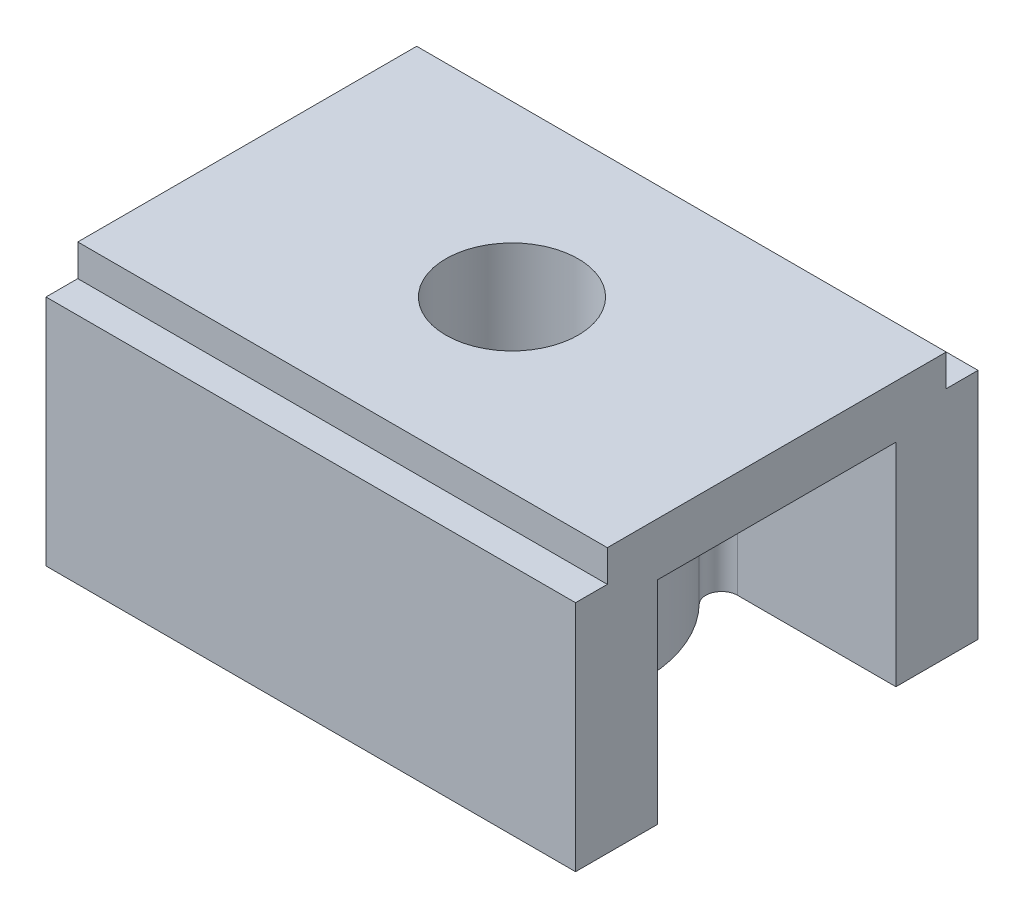
from build123d import *

# Parameters (mm, degrees)
CHANNEL_BODY_DEPTH      = 40
TOP_PLATE_SKETCH_W      = 100
TOP_PLATE_SKETCH_H      = 76
TOP_PLATE_DEPTH         = 10
BORE_SKETCH_R           = 12.5
BORE_25_DEPTH           = 56
GUIDE_GROOVES_SKETCH_W  = 100
GUIDE_GROOVES_SKETCH_H  = 6
GUIDE_GROOVES_6X6_DEPTH = 6


with BuildPart() as part:
    # Channel Profile Sketch → Channel Body (new body)
    with BuildSketch(Plane(origin=(0, 0, 0), x_dir=(1, 0, 0), z_dir=(0, 1, 0))):
        with BuildLine():
            Line((-50, 22.5), (-20.093531297, 22.5))
            ThreePointArc((-20.093531297, 22.5), (-17.330574806, 20.668790584), (-17.940652944, 17.410714286))
            ThreePointArc((-17.940652944, 17.410714286), (-25, 0), (-17.940652944, -17.410714286))
            ThreePointArc((-17.940652944, -17.410714286), (-17.330574806, -20.668790584), (-20.093531297, -22.5))
            Line((-20.093531297, -22.5), (-50, -22.5))
            Line((-50, -22.5), (-50, -38))
            Line((-50, -38), (50, -38))
            Line((50, -38), (50, -22.5))
            Line((50, -22.5), (20.093531297, -22.5))
            ThreePointArc((20.093531297, -22.5), (17.330574806, -20.668790584), (17.940652944, -17.410714286))
            ThreePointArc((17.940652944, -17.410714286), (25, 0), (17.940652944, 17.410714286))
            ThreePointArc((17.940652944, 17.410714286), (17.330574806, 20.668790584), (20.093531297, 22.5))
            Line((20.093531297, 22.5), (50, 22.5))
            Line((50, 22.5), (50, 38))
            Line((50, 38), (-50, 38))
            Line((-50, 38), (-50, 22.5))
        make_face()
    extrude(amount=CHANNEL_BODY_DEPTH)

    # Top Plate Sketch → Top Plate (add)
    with BuildSketch(Plane(origin=(0, 40, 0), x_dir=(1, 0, 0), z_dir=(0, 1, 0))):
        Rectangle(TOP_PLATE_SKETCH_W, TOP_PLATE_SKETCH_H)
    extrude(amount=TOP_PLATE_DEPTH)

    # Bore Sketch → Bore Ø25 (cut)
    with BuildSketch(Plane(origin=(0, 50, 0), x_dir=(1, 0, 0), z_dir=(0, 1, 0))):
        with Locations(Location((0, 0, 0), (0, 0, 270))):
            Circle(BORE_SKETCH_R)
    extrude(amount=-BORE_25_DEPTH, mode=Mode.SUBTRACT)

    # Guide Grooves Sketch → Guide Grooves 6x6 (cut)
    with BuildSketch(Plane(origin=(0, 50, 0), x_dir=(1, 0, 0), z_dir=(0, 1, 0))):
        with Locations((0, 35)):
            Rectangle(GUIDE_GROOVES_SKETCH_W, GUIDE_GROOVES_SKETCH_H)
        with Locations((0, -35)):
            Rectangle(GUIDE_GROOVES_SKETCH_W, GUIDE_GROOVES_SKETCH_H)
    extrude(amount=-GUIDE_GROOVES_6X6_DEPTH, mode=Mode.SUBTRACT)


solid = part.part
